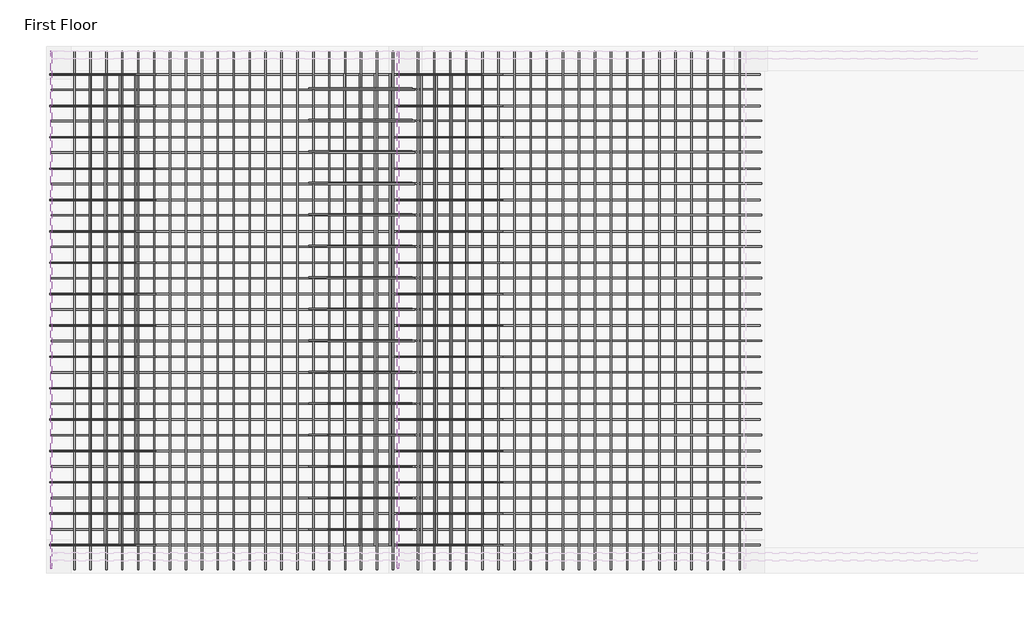
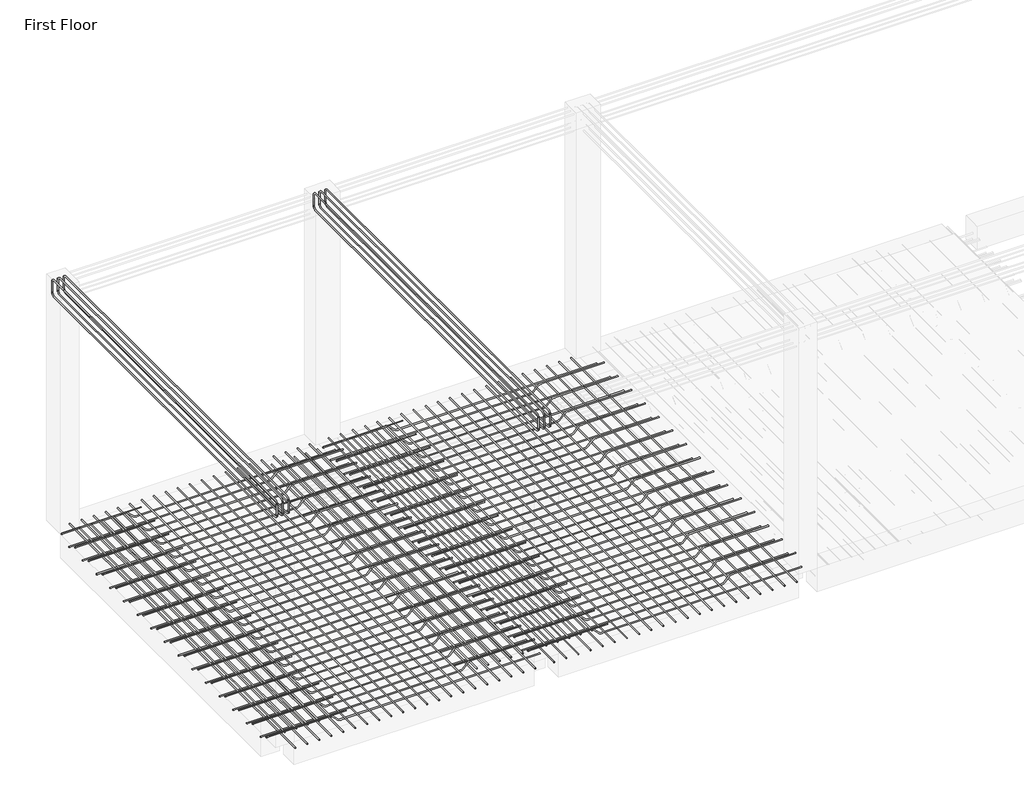
# One storey, part 2 of 4: 16 reinforcing bars.
"""IFC4 building model written with IfcOpenShell, lengths in millimetres."""

from ifc_helpers import new_model, si_unit, point, frame, origin, place, context, project, spatial, polyline, circle_curve, trimmed, segment, composite_curve, source, transform, mapped, element, save
from ifc_brep_helpers import swept_disk

model = new_model("IFC4")

# Units and contexts
model_context = context("Model", 3, world=origin())
ifc_project = project(units=[si_unit("LENGTHUNIT", "METRE", prefix="MILLI")], contexts=[model_context])

# Site, building, storey
site = spatial("IfcSite", under=ifc_project)
building = spatial("IfcBuilding", under=site)
storey = spatial("IfcBuildingStorey", under=building, Name="First Floor", Elevation=3200.4)

# Reinforcing bars
placement = place(None, origin())
reinforcing_bar_shape = source(origin(), model_context, "Body", "SolidModel", [
    swept_disk(composite_curve([segment(polyline([(-9335.8112474, 5017.2334631, 6163.6994949), (-9335.8112474, 5017.2334631, 6311.6994949)]), True, "CONTINUOUS"), segment(trimmed(circle_curve(frame((-9335.8112474, 4971.2334631, 6311.6994949), z_axis=(1.0, 0.0, 0.0), x_axis=(0.0, 46.0, 0.0)), 46.0), [point((-9335.8112474, 5017.2334631, 6311.6994949))], [point((-9335.8112474, 4971.2334631, 6357.6994949))], True, "CARTESIAN"), True, "CONTINUOUS"), segment(polyline([(-9335.8112474, 4971.2334631, 6357.6994949), (-9335.8112474, 278.4334631, 6357.6994949)]), True, "CONTINUOUS"), segment(trimmed(circle_curve(frame((-9335.8112474, 278.4334631, 6311.6994949), z_axis=(1.0, 0.0, 0.0), x_axis=(0.0, 0.0, 46.0)), 46.0), [point((-9335.8112474, 278.4334631, 6357.6994949))], [point((-9335.8112474, 232.4334631, 6311.6994949))], True, "CARTESIAN"), True, "CONTINUOUS"), segment(polyline([(-9335.8112474, 232.4334631, 6311.6994949), (-9335.8112474, 232.4334631, 6163.6994949)]), True, "CONTINUOUS")], self_intersect=False), 6.0),
])
element("IfcReinforcingBar", 1, at=placement, inside=storey, context=model_context, shape_type="MappedRepresentation", body=[
    mapped(reinforcing_bar_shape, transform((0.0, 0.0, 0.0), x_axis=(1.0, 0.0, 0.0), y_axis=(0.0, 1.0, 0.0), z_axis=(0.0, 0.0, 1.0))),
    mapped(reinforcing_bar_shape, transform((71.1994949, 0.0, 0.0), x_axis=(1.0, 0.0, 0.0), y_axis=(0.0, 1.0, 0.0), z_axis=(0.0, 0.0, 1.0))),
    mapped(reinforcing_bar_shape, transform((142.3989899, 0.0, 0.0), x_axis=(1.0, 0.0, 0.0), y_axis=(0.0, 1.0, 0.0), z_axis=(0.0, 0.0, 1.0))),
])
reinforcing_bar_2_shape = source(origin(), model_context, "Body", "SolidModel", [
    swept_disk(composite_curve([segment(polyline([(-9335.8112474, 5017.2334631, 6333.1005051), (-9335.8112474, 5017.2334631, 6185.1005051)]), True, "CONTINUOUS"), segment(trimmed(circle_curve(frame((-9335.8112474, 4971.2334631, 6185.1005051), z_axis=(-1.0, 0.0, 0.0), x_axis=(0.0, 46.0, 0.0)), 46.0), [point((-9335.8112474, 5017.2334631, 6185.1005051))], [point((-9335.8112474, 4971.2334631, 6139.1005051))], True, "CARTESIAN"), True, "CONTINUOUS"), segment(polyline([(-9335.8112474, 4971.2334631, 6139.1005051), (-9335.8112474, 278.4334631, 6139.1005051)]), True, "CONTINUOUS"), segment(trimmed(circle_curve(frame((-9335.8112474, 278.4334631, 6185.1005051), z_axis=(-1.0, 0.0, 0.0), x_axis=(0.0, 0.0, -46.0)), 46.0), [point((-9335.8112474, 278.4334631, 6139.1005051))], [point((-9335.8112474, 232.4334631, 6185.1005051))], True, "CARTESIAN"), True, "CONTINUOUS"), segment(polyline([(-9335.8112474, 232.4334631, 6185.1005051), (-9335.8112474, 232.4334631, 6333.1005051)]), True, "CONTINUOUS")], self_intersect=False), 6.0),
])
element("IfcReinforcingBar", 2, at=placement, inside=storey, context=model_context, shape_type="MappedRepresentation", body=[
    mapped(reinforcing_bar_2_shape, transform((0.0, 0.0, 0.0), x_axis=(1.0, 0.0, 0.0), y_axis=(0.0, 1.0, 0.0), z_axis=(0.0, 0.0, 1.0))),
    mapped(reinforcing_bar_2_shape, transform((71.1994949, 0.0, 0.0), x_axis=(1.0, 0.0, 0.0), y_axis=(0.0, 1.0, 0.0), z_axis=(0.0, 0.0, 1.0))),
    mapped(reinforcing_bar_2_shape, transform((142.3989899, 0.0, 0.0), x_axis=(1.0, 0.0, 0.0), y_axis=(0.0, 1.0, 0.0), z_axis=(0.0, 0.0, 1.0))),
])
reinforcing_bar_3_shape = source(origin(), model_context, "Body", "SolidModel", [
    swept_disk(composite_curve([segment(polyline([(-6122.7112474, 5017.2334631, 6163.6994949), (-6122.7112474, 5017.2334631, 6311.6994949)]), True, "CONTINUOUS"), segment(trimmed(circle_curve(frame((-6122.7112474, 4971.2334631, 6311.6994949), z_axis=(1.0, 0.0, 0.0), x_axis=(0.0, 46.0, 0.0)), 46.0), [point((-6122.7112474, 5017.2334631, 6311.6994949))], [point((-6122.7112474, 4971.2334631, 6357.6994949))], True, "CARTESIAN"), True, "CONTINUOUS"), segment(polyline([(-6122.7112474, 4971.2334631, 6357.6994949), (-6122.7112474, 278.4334631, 6357.6994949)]), True, "CONTINUOUS"), segment(trimmed(circle_curve(frame((-6122.7112474, 278.4334631, 6311.6994949), z_axis=(1.0, 0.0, 0.0), x_axis=(0.0, 0.0, 46.0)), 46.0), [point((-6122.7112474, 278.4334631, 6357.6994949))], [point((-6122.7112474, 232.4334631, 6311.6994949))], True, "CARTESIAN"), True, "CONTINUOUS"), segment(polyline([(-6122.7112474, 232.4334631, 6311.6994949), (-6122.7112474, 232.4334631, 6163.6994949)]), True, "CONTINUOUS")], self_intersect=False), 6.0),
])
element("IfcReinforcingBar", 3, at=placement, inside=storey, context=model_context, shape_type="MappedRepresentation", body=[
    mapped(reinforcing_bar_3_shape, transform((0.0, 0.0, 0.0), x_axis=(1.0, 0.0, 0.0), y_axis=(0.0, 1.0, 0.0), z_axis=(0.0, 0.0, 1.0))),
    mapped(reinforcing_bar_3_shape, transform((71.1994949, 0.0, 0.0), x_axis=(1.0, 0.0, 0.0), y_axis=(0.0, 1.0, 0.0), z_axis=(0.0, 0.0, 1.0))),
    mapped(reinforcing_bar_3_shape, transform((142.3989899, 0.0, 0.0), x_axis=(1.0, 0.0, 0.0), y_axis=(0.0, 1.0, 0.0), z_axis=(0.0, 0.0, 1.0))),
])
reinforcing_bar_4_shape = source(origin(), model_context, "Body", "SolidModel", [
    swept_disk(composite_curve([segment(polyline([(-6122.7112474, 5017.2334631, 6333.1005051), (-6122.7112474, 5017.2334631, 6185.1005051)]), True, "CONTINUOUS"), segment(trimmed(circle_curve(frame((-6122.7112474, 4971.2334631, 6185.1005051), z_axis=(-1.0, 0.0, 0.0), x_axis=(0.0, 46.0, 0.0)), 46.0), [point((-6122.7112474, 5017.2334631, 6185.1005051))], [point((-6122.7112474, 4971.2334631, 6139.1005051))], True, "CARTESIAN"), True, "CONTINUOUS"), segment(polyline([(-6122.7112474, 4971.2334631, 6139.1005051), (-6122.7112474, 278.4334631, 6139.1005051)]), True, "CONTINUOUS"), segment(trimmed(circle_curve(frame((-6122.7112474, 278.4334631, 6185.1005051), z_axis=(-1.0, 0.0, 0.0), x_axis=(0.0, 0.0, -46.0)), 46.0), [point((-6122.7112474, 278.4334631, 6139.1005051))], [point((-6122.7112474, 232.4334631, 6185.1005051))], True, "CARTESIAN"), True, "CONTINUOUS"), segment(polyline([(-6122.7112474, 232.4334631, 6185.1005051), (-6122.7112474, 232.4334631, 6333.1005051)]), True, "CONTINUOUS")], self_intersect=False), 6.0),
])
element("IfcReinforcingBar", 4, at=placement, inside=storey, context=model_context, shape_type="MappedRepresentation", body=[
    mapped(reinforcing_bar_4_shape, transform((0.0, 0.0, 0.0), x_axis=(1.0, 0.0, 0.0), y_axis=(0.0, 1.0, 0.0), z_axis=(0.0, 0.0, 1.0))),
    mapped(reinforcing_bar_4_shape, transform((71.1994949, 0.0, 0.0), x_axis=(1.0, 0.0, 0.0), y_axis=(0.0, 1.0, 0.0), z_axis=(0.0, 0.0, 1.0))),
    mapped(reinforcing_bar_4_shape, transform((142.3989899, 0.0, 0.0), x_axis=(1.0, 0.0, 0.0), y_axis=(0.0, 1.0, 0.0), z_axis=(0.0, 0.0, 1.0))),
])
reinforcing_bar_5_shape = source(origin(), model_context, "Body", "SolidModel", [
    swept_disk(composite_curve([segment(polyline([(-9347.5125695, 4803.6334631, 3169.4), (-8565.5792829, 4803.6334631, 3169.4)]), True, "CONTINUOUS"), segment(trimmed(circle_curve(frame((-8565.5792829, 4803.6334631, 3123.4), z_axis=(0.0, 1.0, 0.0), x_axis=(0.0, 0.0, 46.0)), 46.0), [point((-8565.5792829, 4803.6334631, 3169.4))], [point((-8533.052371, 4803.6334631, 3155.9269119))], True, "CARTESIAN"), True, "CONTINUOUS"), segment(polyline([(-8533.052371, 4803.6334631, 3155.9269119), (-8469.5985471, 4803.6334631, 3092.4730881)]), True, "CONTINUOUS"), segment(trimmed(circle_curve(frame((-8437.0716352, 4803.6334631, 3125.0), z_axis=(0.0, -1.0000000000000002, 0.0), x_axis=(-32.526911900000414, 0.0, -32.52691189999996)), 46.0), [point((-8469.5985471, 4803.6334631, 3092.4730881))], [point((-8437.0716352, 4803.6334631, 3079.0))], True, "CARTESIAN"), True, "CONTINUOUS"), segment(polyline([(-8437.0716352, 4803.6334631, 3079.0), (-5982.0597449, 4803.6334631, 3079.0)]), True, "CONTINUOUS")], self_intersect=False), 6.0),
])
element("IfcReinforcingBar", 5, at=placement, inside=storey, context=model_context, shape_type="MappedRepresentation", body=[
    mapped(reinforcing_bar_5_shape, transform((0.0, 0.0, 0.0), x_axis=(1.0, 0.0, 0.0), y_axis=(0.0, 1.0, 0.0), z_axis=(0.0, 0.0, 1.0))),
    mapped(reinforcing_bar_5_shape, transform((0.0, -290.5066667, 0.0), x_axis=(1.0, 0.0, 0.0), y_axis=(0.0, 1.0, 0.0), z_axis=(0.0, 0.0, 1.0))),
    mapped(reinforcing_bar_5_shape, transform((0.0, -581.0133333, 0.0), x_axis=(1.0, 0.0, 0.0), y_axis=(0.0, 1.0, 0.0), z_axis=(0.0, 0.0, 1.0))),
    mapped(reinforcing_bar_5_shape, transform((0.0, -871.52, 0.0), x_axis=(1.0, 0.0, 0.0), y_axis=(0.0, 1.0, 0.0), z_axis=(0.0, 0.0, 1.0))),
    mapped(reinforcing_bar_5_shape, transform((0.0, -1162.0266667, 0.0), x_axis=(1.0, 0.0, 0.0), y_axis=(0.0, 1.0, 0.0), z_axis=(0.0, 0.0, 1.0))),
    mapped(reinforcing_bar_5_shape, transform((0.0, -1452.5333333, 0.0), x_axis=(1.0, 0.0, 0.0), y_axis=(0.0, 1.0, 0.0), z_axis=(0.0, 0.0, 1.0))),
    mapped(reinforcing_bar_5_shape, transform((0.0, -1743.04, 0.0), x_axis=(1.0, 0.0, 0.0), y_axis=(0.0, 1.0, 0.0), z_axis=(0.0, 0.0, 1.0))),
    mapped(reinforcing_bar_5_shape, transform((0.0, -2033.5466667, 0.0), x_axis=(1.0, 0.0, 0.0), y_axis=(0.0, 1.0, 0.0), z_axis=(0.0, 0.0, 1.0))),
    mapped(reinforcing_bar_5_shape, transform((0.0, -2324.0533333, 0.0), x_axis=(1.0, 0.0, 0.0), y_axis=(0.0, 1.0, 0.0), z_axis=(0.0, 0.0, 1.0))),
    mapped(reinforcing_bar_5_shape, transform((0.0, -2614.56, 0.0), x_axis=(1.0, 0.0, 0.0), y_axis=(0.0, 1.0, 0.0), z_axis=(0.0, 0.0, 1.0))),
    mapped(reinforcing_bar_5_shape, transform((0.0, -2905.0666667, 0.0), x_axis=(1.0, 0.0, 0.0), y_axis=(0.0, 1.0, 0.0), z_axis=(0.0, 0.0, 1.0))),
    mapped(reinforcing_bar_5_shape, transform((0.0, -3195.5733333, 0.0), x_axis=(1.0, 0.0, 0.0), y_axis=(0.0, 1.0, 0.0), z_axis=(0.0, 0.0, 1.0))),
    mapped(reinforcing_bar_5_shape, transform((0.0, -3486.08, 0.0), x_axis=(1.0, 0.0, 0.0), y_axis=(0.0, 1.0, 0.0), z_axis=(0.0, 0.0, 1.0))),
    mapped(reinforcing_bar_5_shape, transform((0.0, -3776.5866667, 0.0), x_axis=(1.0, 0.0, 0.0), y_axis=(0.0, 1.0, 0.0), z_axis=(0.0, 0.0, 1.0))),
    mapped(reinforcing_bar_5_shape, transform((0.0, -4067.0933333, 0.0), x_axis=(1.0, 0.0, 0.0), y_axis=(0.0, 1.0, 0.0), z_axis=(0.0, 0.0, 1.0))),
    mapped(reinforcing_bar_5_shape, transform((0.0, -4357.6, 0.0), x_axis=(1.0, 0.0, 0.0), y_axis=(0.0, 1.0, 0.0), z_axis=(0.0, 0.0, 1.0))),
])
reinforcing_bar_6_shape = source(origin(), model_context, "Body", "SolidModel", [
    swept_disk(composite_curve([segment(polyline([(-5968.6109354, 590.4513536, 3169.4), (-6750.544222, 590.4513536, 3169.4)]), True, "CONTINUOUS"), segment(trimmed(circle_curve(frame((-6750.544222, 590.4513536, 3123.4), z_axis=(0.0, -1.0, 0.0), x_axis=(0.0, 0.0, 46.0)), 46.0), [point((-6750.544222, 590.4513536, 3169.4))], [point((-6783.0711339, 590.4513536, 3155.9269119))], True, "CARTESIAN"), True, "CONTINUOUS"), segment(polyline([(-6783.0711339, 590.4513536, 3155.9269119), (-6846.5249578, 590.4513536, 3092.4730881)]), True, "CONTINUOUS"), segment(trimmed(circle_curve(frame((-6879.0518697, 590.4513536, 3125.0), z_axis=(0.0, 1.0000000000000002, 0.0), x_axis=(32.526911899999504, 0.0, -32.52691189999996)), 46.0), [point((-6846.5249578, 590.4513536, 3092.4730881))], [point((-6879.0518697, 590.4513536, 3079.0))], True, "CARTESIAN"), True, "CONTINUOUS"), segment(polyline([(-6879.0518697, 590.4513536, 3079.0), (-9334.06376, 590.4513536, 3079.0)]), True, "CONTINUOUS")], self_intersect=False), 6.0),
])
element("IfcReinforcingBar", 6, at=placement, inside=storey, context=model_context, shape_type="MappedRepresentation", body=[
    mapped(reinforcing_bar_6_shape, transform((0.0, 0.0, 0.0), x_axis=(1.0, 0.0, 0.0), y_axis=(0.0, 1.0, 0.0), z_axis=(0.0, 0.0, 1.0))),
    mapped(reinforcing_bar_6_shape, transform((0.0, 290.9296088, 0.0), x_axis=(1.0, 0.0, 0.0), y_axis=(0.0, 1.0, 0.0), z_axis=(0.0, 0.0, 1.0))),
    mapped(reinforcing_bar_6_shape, transform((0.0, 581.8592177, 0.0), x_axis=(1.0, 0.0, 0.0), y_axis=(0.0, 1.0, 0.0), z_axis=(0.0, 0.0, 1.0))),
    mapped(reinforcing_bar_6_shape, transform((0.0, 872.7888265, 0.0), x_axis=(1.0, 0.0, 0.0), y_axis=(0.0, 1.0, 0.0), z_axis=(0.0, 0.0, 1.0))),
    mapped(reinforcing_bar_6_shape, transform((0.0, 1163.7184353, 0.0), x_axis=(1.0, 0.0, 0.0), y_axis=(0.0, 1.0, 0.0), z_axis=(0.0, 0.0, 1.0))),
    mapped(reinforcing_bar_6_shape, transform((0.0, 1454.6480442, 0.0), x_axis=(1.0, 0.0, 0.0), y_axis=(0.0, 1.0, 0.0), z_axis=(0.0, 0.0, 1.0))),
    mapped(reinforcing_bar_6_shape, transform((0.0, 1745.577653, 0.0), x_axis=(1.0, 0.0, 0.0), y_axis=(0.0, 1.0, 0.0), z_axis=(0.0, 0.0, 1.0))),
    mapped(reinforcing_bar_6_shape, transform((0.0, 2036.5072618, 0.0), x_axis=(1.0, 0.0, 0.0), y_axis=(0.0, 1.0, 0.0), z_axis=(0.0, 0.0, 1.0))),
    mapped(reinforcing_bar_6_shape, transform((0.0, 2327.4368707, 0.0), x_axis=(1.0, 0.0, 0.0), y_axis=(0.0, 1.0, 0.0), z_axis=(0.0, 0.0, 1.0))),
    mapped(reinforcing_bar_6_shape, transform((0.0, 2618.3664795, 0.0), x_axis=(1.0, 0.0, 0.0), y_axis=(0.0, 1.0, 0.0), z_axis=(0.0, 0.0, 1.0))),
    mapped(reinforcing_bar_6_shape, transform((0.0, 2909.2960883, 0.0), x_axis=(1.0, 0.0, 0.0), y_axis=(0.0, 1.0, 0.0), z_axis=(0.0, 0.0, 1.0))),
    mapped(reinforcing_bar_6_shape, transform((0.0, 3200.2256972, 0.0), x_axis=(1.0, 0.0, 0.0), y_axis=(0.0, 1.0, 0.0), z_axis=(0.0, 0.0, 1.0))),
    mapped(reinforcing_bar_6_shape, transform((0.0, 3491.155306, 0.0), x_axis=(1.0, 0.0, 0.0), y_axis=(0.0, 1.0, 0.0), z_axis=(0.0, 0.0, 1.0))),
    mapped(reinforcing_bar_6_shape, transform((0.0, 3782.0849148, 0.0), x_axis=(1.0, 0.0, 0.0), y_axis=(0.0, 1.0, 0.0), z_axis=(0.0, 0.0, 1.0))),
    mapped(reinforcing_bar_6_shape, transform((0.0, 4073.0145236, 0.0), x_axis=(1.0, 0.0, 0.0), y_axis=(0.0, 1.0, 0.0), z_axis=(0.0, 0.0, 1.0))),
])
reinforcing_bar_7_shape = source(origin(), model_context, "Body", "SolidModel", [
    swept_disk(composite_curve([segment(polyline([(-8556.5984173, 4809.6334631, 3159.1006995), (-8556.5984173, 440.0334631, 3159.1006995)]), True, "CONTINUOUS")], self_intersect=False), 6.0),
])
element("IfcReinforcingBar", 7, at=placement, inside=storey, context=model_context, shape_type="MappedRepresentation", body=[
    mapped(reinforcing_bar_7_shape, transform((0.0, 0.0, 0.0), x_axis=(1.0, 0.0, 0.0), y_axis=(0.0, 1.0, 0.0), z_axis=(0.0, 0.0, 1.0))),
    mapped(reinforcing_bar_7_shape, transform((-140.6783338, 0.0, 0.0), x_axis=(1.0, 0.0, 0.0), y_axis=(0.0, 1.0, 0.0), z_axis=(0.0, 0.0, 1.0))),
    mapped(reinforcing_bar_7_shape, transform((-281.3566676, 0.0, 0.0), x_axis=(1.0, 0.0, 0.0), y_axis=(0.0, 1.0, 0.0), z_axis=(0.0, 0.0, 1.0))),
    mapped(reinforcing_bar_7_shape, transform((-422.0350014, 0.0, 0.0), x_axis=(1.0, 0.0, 0.0), y_axis=(0.0, 1.0, 0.0), z_axis=(0.0, 0.0, 1.0))),
    mapped(reinforcing_bar_7_shape, transform((-562.7133352, 0.0, 0.0), x_axis=(1.0, 0.0, 0.0), y_axis=(0.0, 1.0, 0.0), z_axis=(0.0, 0.0, 1.0))),
])
reinforcing_bar_8_shape = source(origin(), model_context, "Body", "SolidModel", [
    swept_disk(composite_curve([segment(polyline([(-6759.5250876, 4809.6334631, 3159.1006995), (-6759.5250876, 440.0334631, 3159.1006995)]), True, "CONTINUOUS")], self_intersect=False), 6.0),
])
element("IfcReinforcingBar", 8, at=placement, inside=storey, context=model_context, shape_type="MappedRepresentation", body=[
    mapped(reinforcing_bar_8_shape, transform((0.0, 0.0, 0.0), x_axis=(1.0, 0.0, 0.0), y_axis=(0.0, 1.0, 0.0), z_axis=(0.0, 0.0, 1.0))),
    mapped(reinforcing_bar_8_shape, transform((140.6783338, 0.0, 0.0), x_axis=(1.0, 0.0, 0.0), y_axis=(0.0, 1.0, 0.0), z_axis=(0.0, 0.0, 1.0))),
    mapped(reinforcing_bar_8_shape, transform((281.3566676, 0.0, 0.0), x_axis=(1.0, 0.0, 0.0), y_axis=(0.0, 1.0, 0.0), z_axis=(0.0, 0.0, 1.0))),
    mapped(reinforcing_bar_8_shape, transform((422.0350014, 0.0, 0.0), x_axis=(1.0, 0.0, 0.0), y_axis=(0.0, 1.0, 0.0), z_axis=(0.0, 0.0, 1.0))),
    mapped(reinforcing_bar_8_shape, transform((562.7133352, 0.0, 0.0), x_axis=(1.0, 0.0, 0.0), y_axis=(0.0, 1.0, 0.0), z_axis=(0.0, 0.0, 1.0))),
])
reinforcing_bar_9_shape = source(origin(), model_context, "Body", "SolidModel", [
    swept_disk(composite_curve([segment(polyline([(-9338.4522926, 4805.6334631, 3171.4), (-8365.7369752, 4805.6334631, 3171.4)]), True, "CONTINUOUS")], self_intersect=False), 4.0),
])
element("IfcReinforcingBar", 9, at=placement, inside=storey, context=model_context, shape_type="MappedRepresentation", body=[
    mapped(reinforcing_bar_9_shape, transform((0.0, 0.0, 0.0), x_axis=(1.0, 0.0, 0.0), y_axis=(0.0, 1.0, 0.0), z_axis=(0.0, 0.0, 1.0))),
    mapped(reinforcing_bar_9_shape, transform((0.0, -290.7733333, 0.0), x_axis=(1.0, 0.0, 0.0), y_axis=(0.0, 1.0, 0.0), z_axis=(0.0, 0.0, 1.0))),
    mapped(reinforcing_bar_9_shape, transform((0.0, -581.5466667, 0.0), x_axis=(1.0, 0.0, 0.0), y_axis=(0.0, 1.0, 0.0), z_axis=(0.0, 0.0, 1.0))),
    mapped(reinforcing_bar_9_shape, transform((0.0, -872.32, 0.0), x_axis=(1.0, 0.0, 0.0), y_axis=(0.0, 1.0, 0.0), z_axis=(0.0, 0.0, 1.0))),
    mapped(reinforcing_bar_9_shape, transform((0.0, -1163.0933333, 0.0), x_axis=(1.0, 0.0, 0.0), y_axis=(0.0, 1.0, 0.0), z_axis=(0.0, 0.0, 1.0))),
    mapped(reinforcing_bar_9_shape, transform((0.0, -1453.8666667, 0.0), x_axis=(1.0, 0.0, 0.0), y_axis=(0.0, 1.0, 0.0), z_axis=(0.0, 0.0, 1.0))),
    mapped(reinforcing_bar_9_shape, transform((0.0, -1744.64, 0.0), x_axis=(1.0, 0.0, 0.0), y_axis=(0.0, 1.0, 0.0), z_axis=(0.0, 0.0, 1.0))),
    mapped(reinforcing_bar_9_shape, transform((0.0, -2035.4133333, 0.0), x_axis=(1.0, 0.0, 0.0), y_axis=(0.0, 1.0, 0.0), z_axis=(0.0, 0.0, 1.0))),
    mapped(reinforcing_bar_9_shape, transform((0.0, -2326.1866667, 0.0), x_axis=(1.0, 0.0, 0.0), y_axis=(0.0, 1.0, 0.0), z_axis=(0.0, 0.0, 1.0))),
    mapped(reinforcing_bar_9_shape, transform((0.0, -2616.96, 0.0), x_axis=(1.0, 0.0, 0.0), y_axis=(0.0, 1.0, 0.0), z_axis=(0.0, 0.0, 1.0))),
    mapped(reinforcing_bar_9_shape, transform((0.0, -2907.7333333, 0.0), x_axis=(1.0, 0.0, 0.0), y_axis=(0.0, 1.0, 0.0), z_axis=(0.0, 0.0, 1.0))),
    mapped(reinforcing_bar_9_shape, transform((0.0, -3198.5066667, 0.0), x_axis=(1.0, 0.0, 0.0), y_axis=(0.0, 1.0, 0.0), z_axis=(0.0, 0.0, 1.0))),
    mapped(reinforcing_bar_9_shape, transform((0.0, -3489.28, 0.0), x_axis=(1.0, 0.0, 0.0), y_axis=(0.0, 1.0, 0.0), z_axis=(0.0, 0.0, 1.0))),
    mapped(reinforcing_bar_9_shape, transform((0.0, -3780.0533333, 0.0), x_axis=(1.0, 0.0, 0.0), y_axis=(0.0, 1.0, 0.0), z_axis=(0.0, 0.0, 1.0))),
    mapped(reinforcing_bar_9_shape, transform((0.0, -4070.8266667, 0.0), x_axis=(1.0, 0.0, 0.0), y_axis=(0.0, 1.0, 0.0), z_axis=(0.0, 0.0, 1.0))),
    mapped(reinforcing_bar_9_shape, transform((0.0, -4361.6, 0.0), x_axis=(1.0, 0.0, 0.0), y_axis=(0.0, 1.0, 0.0), z_axis=(0.0, 0.0, 1.0))),
])
reinforcing_bar_10_shape = source(origin(), model_context, "Body", "SolidModel", [
    swept_disk(composite_curve([segment(polyline([(-5991.3123639, 4678.4115375, 3171.4), (-6950.3865297, 4678.4115375, 3171.4)]), True, "CONTINUOUS")], self_intersect=False), 4.0),
])
element("IfcReinforcingBar", 10, at=placement, inside=storey, context=model_context, shape_type="MappedRepresentation", body=[
    mapped(reinforcing_bar_10_shape, transform((0.0, 0.0, 0.0), x_axis=(1.0, 0.0, 0.0), y_axis=(0.0, 1.0, 0.0), z_axis=(0.0, 0.0, 1.0))),
    mapped(reinforcing_bar_10_shape, transform((0.0, -291.8025106, 0.0), x_axis=(1.0, 0.0, 0.0), y_axis=(0.0, 1.0, 0.0), z_axis=(0.0, 0.0, 1.0))),
    mapped(reinforcing_bar_10_shape, transform((0.0, -583.6050212, 0.0), x_axis=(1.0, 0.0, 0.0), y_axis=(0.0, 1.0, 0.0), z_axis=(0.0, 0.0, 1.0))),
    mapped(reinforcing_bar_10_shape, transform((0.0, -875.4075319, 0.0), x_axis=(1.0, 0.0, 0.0), y_axis=(0.0, 1.0, 0.0), z_axis=(0.0, 0.0, 1.0))),
    mapped(reinforcing_bar_10_shape, transform((0.0, -1167.2100425, 0.0), x_axis=(1.0, 0.0, 0.0), y_axis=(0.0, 1.0, 0.0), z_axis=(0.0, 0.0, 1.0))),
    mapped(reinforcing_bar_10_shape, transform((0.0, -1459.0125531, 0.0), x_axis=(1.0, 0.0, 0.0), y_axis=(0.0, 1.0, 0.0), z_axis=(0.0, 0.0, 1.0))),
    mapped(reinforcing_bar_10_shape, transform((0.0, -1750.8150637, 0.0), x_axis=(1.0, 0.0, 0.0), y_axis=(0.0, 1.0, 0.0), z_axis=(0.0, 0.0, 1.0))),
    mapped(reinforcing_bar_10_shape, transform((0.0, -2042.6175743, 0.0), x_axis=(1.0, 0.0, 0.0), y_axis=(0.0, 1.0, 0.0), z_axis=(0.0, 0.0, 1.0))),
    mapped(reinforcing_bar_10_shape, transform((0.0, -2334.420085, 0.0), x_axis=(1.0, 0.0, 0.0), y_axis=(0.0, 1.0, 0.0), z_axis=(0.0, 0.0, 1.0))),
    mapped(reinforcing_bar_10_shape, transform((0.0, -2626.2225956, 0.0), x_axis=(1.0, 0.0, 0.0), y_axis=(0.0, 1.0, 0.0), z_axis=(0.0, 0.0, 1.0))),
    mapped(reinforcing_bar_10_shape, transform((0.0, -2918.0251062, 0.0), x_axis=(1.0, 0.0, 0.0), y_axis=(0.0, 1.0, 0.0), z_axis=(0.0, 0.0, 1.0))),
    mapped(reinforcing_bar_10_shape, transform((0.0, -3209.8276168, 0.0), x_axis=(1.0, 0.0, 0.0), y_axis=(0.0, 1.0, 0.0), z_axis=(0.0, 0.0, 1.0))),
    mapped(reinforcing_bar_10_shape, transform((0.0, -3501.6301274, 0.0), x_axis=(1.0, 0.0, 0.0), y_axis=(0.0, 1.0, 0.0), z_axis=(0.0, 0.0, 1.0))),
    mapped(reinforcing_bar_10_shape, transform((0.0, -3793.4326381, 0.0), x_axis=(1.0, 0.0, 0.0), y_axis=(0.0, 1.0, 0.0), z_axis=(0.0, 0.0, 1.0))),
    mapped(reinforcing_bar_10_shape, transform((0.0, -4085.2351487, 0.0), x_axis=(1.0, 0.0, 0.0), y_axis=(0.0, 1.0, 0.0), z_axis=(0.0, 0.0, 1.0))),
])
reinforcing_bar_11_shape = source(origin(), model_context, "Body", "SolidModel", [
    swept_disk(composite_curve([segment(polyline([(-6169.8117524, 218.9117605, 3087.5387401), (-6169.8117524, 5019.9992064, 3087.5387401)]), True, "CONTINUOUS")], self_intersect=False), 6.0),
])
element("IfcReinforcingBar", 11, at=placement, inside=storey, context=model_context, shape_type="MappedRepresentation", body=[
    mapped(reinforcing_bar_11_shape, transform((0.0, 0.0, 0.0), x_axis=(1.0, 0.0, 0.0), y_axis=(0.0, 1.0, 0.0), z_axis=(0.0, 0.0, 1.0))),
    mapped(reinforcing_bar_11_shape, transform((-147.475, 0.0, 0.0), x_axis=(1.0, 0.0, 0.0), y_axis=(0.0, 1.0, 0.0), z_axis=(0.0, 0.0, 1.0))),
    mapped(reinforcing_bar_11_shape, transform((-294.95, 0.0, 0.0), x_axis=(1.0, 0.0, 0.0), y_axis=(0.0, 1.0, 0.0), z_axis=(0.0, 0.0, 1.0))),
    mapped(reinforcing_bar_11_shape, transform((-442.425, 0.0, 0.0), x_axis=(1.0, 0.0, 0.0), y_axis=(0.0, 1.0, 0.0), z_axis=(0.0, 0.0, 1.0))),
    mapped(reinforcing_bar_11_shape, transform((-589.9, 0.0, 0.0), x_axis=(1.0, 0.0, 0.0), y_axis=(0.0, 1.0, 0.0), z_axis=(0.0, 0.0, 1.0))),
    mapped(reinforcing_bar_11_shape, transform((-737.375, 0.0, 0.0), x_axis=(1.0, 0.0, 0.0), y_axis=(0.0, 1.0, 0.0), z_axis=(0.0, 0.0, 1.0))),
    mapped(reinforcing_bar_11_shape, transform((-884.85, 0.0, 0.0), x_axis=(1.0, 0.0, 0.0), y_axis=(0.0, 1.0, 0.0), z_axis=(0.0, 0.0, 1.0))),
    mapped(reinforcing_bar_11_shape, transform((-1032.325, 0.0, 0.0), x_axis=(1.0, 0.0, 0.0), y_axis=(0.0, 1.0, 0.0), z_axis=(0.0, 0.0, 1.0))),
    mapped(reinforcing_bar_11_shape, transform((-1179.8, 0.0, 0.0), x_axis=(1.0, 0.0, 0.0), y_axis=(0.0, 1.0, 0.0), z_axis=(0.0, 0.0, 1.0))),
    mapped(reinforcing_bar_11_shape, transform((-1327.275, 0.0, 0.0), x_axis=(1.0, 0.0, 0.0), y_axis=(0.0, 1.0, 0.0), z_axis=(0.0, 0.0, 1.0))),
    mapped(reinforcing_bar_11_shape, transform((-1474.75, 0.0, 0.0), x_axis=(1.0, 0.0, 0.0), y_axis=(0.0, 1.0, 0.0), z_axis=(0.0, 0.0, 1.0))),
    mapped(reinforcing_bar_11_shape, transform((-1622.225, 0.0, 0.0), x_axis=(1.0, 0.0, 0.0), y_axis=(0.0, 1.0, 0.0), z_axis=(0.0, 0.0, 1.0))),
    mapped(reinforcing_bar_11_shape, transform((-1769.7, 0.0, 0.0), x_axis=(1.0, 0.0, 0.0), y_axis=(0.0, 1.0, 0.0), z_axis=(0.0, 0.0, 1.0))),
    mapped(reinforcing_bar_11_shape, transform((-1917.175, 0.0, 0.0), x_axis=(1.0, 0.0, 0.0), y_axis=(0.0, 1.0, 0.0), z_axis=(0.0, 0.0, 1.0))),
    mapped(reinforcing_bar_11_shape, transform((-2064.65, 0.0, 0.0), x_axis=(1.0, 0.0, 0.0), y_axis=(0.0, 1.0, 0.0), z_axis=(0.0, 0.0, 1.0))),
    mapped(reinforcing_bar_11_shape, transform((-2212.125, 0.0, 0.0), x_axis=(1.0, 0.0, 0.0), y_axis=(0.0, 1.0, 0.0), z_axis=(0.0, 0.0, 1.0))),
    mapped(reinforcing_bar_11_shape, transform((-2359.6, 0.0, 0.0), x_axis=(1.0, 0.0, 0.0), y_axis=(0.0, 1.0, 0.0), z_axis=(0.0, 0.0, 1.0))),
    mapped(reinforcing_bar_11_shape, transform((-2507.075, 0.0, 0.0), x_axis=(1.0, 0.0, 0.0), y_axis=(0.0, 1.0, 0.0), z_axis=(0.0, 0.0, 1.0))),
    mapped(reinforcing_bar_11_shape, transform((-2654.55, 0.0, 0.0), x_axis=(1.0, 0.0, 0.0), y_axis=(0.0, 1.0, 0.0), z_axis=(0.0, 0.0, 1.0))),
    mapped(reinforcing_bar_11_shape, transform((-2802.025, 0.0, 0.0), x_axis=(1.0, 0.0, 0.0), y_axis=(0.0, 1.0, 0.0), z_axis=(0.0, 0.0, 1.0))),
    mapped(reinforcing_bar_11_shape, transform((-2949.5, 0.0, 0.0), x_axis=(1.0, 0.0, 0.0), y_axis=(0.0, 1.0, 0.0), z_axis=(0.0, 0.0, 1.0))),
])
reinforcing_bar_12_shape = source(origin(), model_context, "Body", "SolidModel", [
    swept_disk(composite_curve([segment(polyline([(-6134.4125695, 4803.6334631, 3169.4), (-5352.4792829, 4803.6334631, 3169.4)]), True, "CONTINUOUS"), segment(trimmed(circle_curve(frame((-5352.4792829, 4803.6334631, 3123.4), z_axis=(0.0, 1.0, 0.0), x_axis=(0.0, 0.0, 46.0)), 46.0), [point((-5352.4792829, 4803.6334631, 3169.4))], [point((-5319.952371, 4803.6334631, 3155.9269119))], True, "CARTESIAN"), True, "CONTINUOUS"), segment(polyline([(-5319.952371, 4803.6334631, 3155.9269119), (-5256.4985471, 4803.6334631, 3092.4730881)]), True, "CONTINUOUS"), segment(trimmed(circle_curve(frame((-5223.9716352, 4803.6334631, 3125.0), z_axis=(0.0, -1.0000000000000002, 0.0), x_axis=(-32.526911900000414, 0.0, -32.52691189999996)), 46.0), [point((-5256.4985471, 4803.6334631, 3092.4730881))], [point((-5223.9716352, 4803.6334631, 3079.0))], True, "CARTESIAN"), True, "CONTINUOUS"), segment(polyline([(-5223.9716352, 4803.6334631, 3079.0), (-2768.9597449, 4803.6334631, 3079.0)]), True, "CONTINUOUS")], self_intersect=False), 6.0),
])
element("IfcReinforcingBar", 12, at=placement, inside=storey, context=model_context, shape_type="MappedRepresentation", body=[
    mapped(reinforcing_bar_12_shape, transform((0.0, 0.0, 0.0), x_axis=(1.0, 0.0, 0.0), y_axis=(0.0, 1.0, 0.0), z_axis=(0.0, 0.0, 1.0))),
    mapped(reinforcing_bar_12_shape, transform((0.0, -290.5066667, 0.0), x_axis=(1.0, 0.0, 0.0), y_axis=(0.0, 1.0, 0.0), z_axis=(0.0, 0.0, 1.0))),
    mapped(reinforcing_bar_12_shape, transform((0.0, -581.0133333, 0.0), x_axis=(1.0, 0.0, 0.0), y_axis=(0.0, 1.0, 0.0), z_axis=(0.0, 0.0, 1.0))),
    mapped(reinforcing_bar_12_shape, transform((0.0, -871.52, 0.0), x_axis=(1.0, 0.0, 0.0), y_axis=(0.0, 1.0, 0.0), z_axis=(0.0, 0.0, 1.0))),
    mapped(reinforcing_bar_12_shape, transform((0.0, -1162.0266667, 0.0), x_axis=(1.0, 0.0, 0.0), y_axis=(0.0, 1.0, 0.0), z_axis=(0.0, 0.0, 1.0))),
    mapped(reinforcing_bar_12_shape, transform((0.0, -1452.5333333, 0.0), x_axis=(1.0, 0.0, 0.0), y_axis=(0.0, 1.0, 0.0), z_axis=(0.0, 0.0, 1.0))),
    mapped(reinforcing_bar_12_shape, transform((0.0, -1743.04, 0.0), x_axis=(1.0, 0.0, 0.0), y_axis=(0.0, 1.0, 0.0), z_axis=(0.0, 0.0, 1.0))),
    mapped(reinforcing_bar_12_shape, transform((0.0, -2033.5466667, 0.0), x_axis=(1.0, 0.0, 0.0), y_axis=(0.0, 1.0, 0.0), z_axis=(0.0, 0.0, 1.0))),
    mapped(reinforcing_bar_12_shape, transform((0.0, -2324.0533333, 0.0), x_axis=(1.0, 0.0, 0.0), y_axis=(0.0, 1.0, 0.0), z_axis=(0.0, 0.0, 1.0))),
    mapped(reinforcing_bar_12_shape, transform((0.0, -2614.56, 0.0), x_axis=(1.0, 0.0, 0.0), y_axis=(0.0, 1.0, 0.0), z_axis=(0.0, 0.0, 1.0))),
    mapped(reinforcing_bar_12_shape, transform((0.0, -2905.0666667, 0.0), x_axis=(1.0, 0.0, 0.0), y_axis=(0.0, 1.0, 0.0), z_axis=(0.0, 0.0, 1.0))),
    mapped(reinforcing_bar_12_shape, transform((0.0, -3195.5733333, 0.0), x_axis=(1.0, 0.0, 0.0), y_axis=(0.0, 1.0, 0.0), z_axis=(0.0, 0.0, 1.0))),
    mapped(reinforcing_bar_12_shape, transform((0.0, -3486.08, 0.0), x_axis=(1.0, 0.0, 0.0), y_axis=(0.0, 1.0, 0.0), z_axis=(0.0, 0.0, 1.0))),
    mapped(reinforcing_bar_12_shape, transform((0.0, -3776.5866667, 0.0), x_axis=(1.0, 0.0, 0.0), y_axis=(0.0, 1.0, 0.0), z_axis=(0.0, 0.0, 1.0))),
    mapped(reinforcing_bar_12_shape, transform((0.0, -4067.0933333, 0.0), x_axis=(1.0, 0.0, 0.0), y_axis=(0.0, 1.0, 0.0), z_axis=(0.0, 0.0, 1.0))),
    mapped(reinforcing_bar_12_shape, transform((0.0, -4357.6, 0.0), x_axis=(1.0, 0.0, 0.0), y_axis=(0.0, 1.0, 0.0), z_axis=(0.0, 0.0, 1.0))),
])
reinforcing_bar_13_shape = source(origin(), model_context, "Body", "SolidModel", [
    swept_disk(composite_curve([segment(polyline([(-2755.5109354, 590.4513536, 3169.4), (-3537.444222, 590.4513536, 3169.4)]), True, "CONTINUOUS"), segment(trimmed(circle_curve(frame((-3537.444222, 590.4513536, 3123.4), z_axis=(0.0, -1.0, 0.0), x_axis=(0.0, 0.0, 46.0)), 46.0), [point((-3537.444222, 590.4513536, 3169.4))], [point((-3569.9711339, 590.4513536, 3155.9269119))], True, "CARTESIAN"), True, "CONTINUOUS"), segment(polyline([(-3569.9711339, 590.4513536, 3155.9269119), (-3633.4249578, 590.4513536, 3092.4730881)]), True, "CONTINUOUS"), segment(trimmed(circle_curve(frame((-3665.9518697, 590.4513536, 3125.0), z_axis=(0.0, 1.0000000000000002, 0.0), x_axis=(32.52691189999996, 0.0, -32.52691189999996)), 46.0), [point((-3633.4249578, 590.4513536, 3092.4730881))], [point((-3665.9518697, 590.4513536, 3079.0))], True, "CARTESIAN"), True, "CONTINUOUS"), segment(polyline([(-3665.9518697, 590.4513536, 3079.0), (-6120.96376, 590.4513536, 3079.0)]), True, "CONTINUOUS")], self_intersect=False), 6.0),
])
element("IfcReinforcingBar", 13, at=placement, inside=storey, context=model_context, shape_type="MappedRepresentation", body=[
    mapped(reinforcing_bar_13_shape, transform((0.0, 0.0, 0.0), x_axis=(1.0, 0.0, 0.0), y_axis=(0.0, 1.0, 0.0), z_axis=(0.0, 0.0, 1.0))),
    mapped(reinforcing_bar_13_shape, transform((0.0, 291.2629007, 0.0), x_axis=(1.0, 0.0, 0.0), y_axis=(0.0, 1.0, 0.0), z_axis=(0.0, 0.0, 1.0))),
    mapped(reinforcing_bar_13_shape, transform((0.0, 582.5258014, 0.0), x_axis=(1.0, 0.0, 0.0), y_axis=(0.0, 1.0, 0.0), z_axis=(0.0, 0.0, 1.0))),
    mapped(reinforcing_bar_13_shape, transform((0.0, 873.7887021, 0.0), x_axis=(1.0, 0.0, 0.0), y_axis=(0.0, 1.0, 0.0), z_axis=(0.0, 0.0, 1.0))),
    mapped(reinforcing_bar_13_shape, transform((0.0, 1165.0516028, 0.0), x_axis=(1.0, 0.0, 0.0), y_axis=(0.0, 1.0, 0.0), z_axis=(0.0, 0.0, 1.0))),
    mapped(reinforcing_bar_13_shape, transform((0.0, 1456.3145035, 0.0), x_axis=(1.0, 0.0, 0.0), y_axis=(0.0, 1.0, 0.0), z_axis=(0.0, 0.0, 1.0))),
    mapped(reinforcing_bar_13_shape, transform((0.0, 1747.5774042, 0.0), x_axis=(1.0, 0.0, 0.0), y_axis=(0.0, 1.0, 0.0), z_axis=(0.0, 0.0, 1.0))),
    mapped(reinforcing_bar_13_shape, transform((0.0, 2038.8403049, 0.0), x_axis=(1.0, 0.0, 0.0), y_axis=(0.0, 1.0, 0.0), z_axis=(0.0, 0.0, 1.0))),
    mapped(reinforcing_bar_13_shape, transform((0.0, 2330.1032056, 0.0), x_axis=(1.0, 0.0, 0.0), y_axis=(0.0, 1.0, 0.0), z_axis=(0.0, 0.0, 1.0))),
    mapped(reinforcing_bar_13_shape, transform((0.0, 2621.3661063, 0.0), x_axis=(1.0, 0.0, 0.0), y_axis=(0.0, 1.0, 0.0), z_axis=(0.0, 0.0, 1.0))),
    mapped(reinforcing_bar_13_shape, transform((0.0, 2912.629007, 0.0), x_axis=(1.0, 0.0, 0.0), y_axis=(0.0, 1.0, 0.0), z_axis=(0.0, 0.0, 1.0))),
    mapped(reinforcing_bar_13_shape, transform((0.0, 3203.8919077, 0.0), x_axis=(1.0, 0.0, 0.0), y_axis=(0.0, 1.0, 0.0), z_axis=(0.0, 0.0, 1.0))),
    mapped(reinforcing_bar_13_shape, transform((0.0, 3495.1548084, 0.0), x_axis=(1.0, 0.0, 0.0), y_axis=(0.0, 1.0, 0.0), z_axis=(0.0, 0.0, 1.0))),
    mapped(reinforcing_bar_13_shape, transform((0.0, 3786.4177091, 0.0), x_axis=(1.0, 0.0, 0.0), y_axis=(0.0, 1.0, 0.0), z_axis=(0.0, 0.0, 1.0))),
    mapped(reinforcing_bar_13_shape, transform((0.0, 4077.6806098, 0.0), x_axis=(1.0, 0.0, 0.0), y_axis=(0.0, 1.0, 0.0), z_axis=(0.0, 0.0, 1.0))),
])
reinforcing_bar_14_shape = source(origin(), model_context, "Body", "SolidModel", [
    swept_disk(composite_curve([segment(polyline([(-6125.3522926, 4805.6334631, 3171.4), (-5152.6369752, 4805.6334631, 3171.4)]), True, "CONTINUOUS")], self_intersect=False), 4.0),
])
element("IfcReinforcingBar", 14, at=placement, inside=storey, context=model_context, shape_type="MappedRepresentation", body=[
    mapped(reinforcing_bar_14_shape, transform((0.0, 0.0, 0.0), x_axis=(1.0, 0.0, 0.0), y_axis=(0.0, 1.0, 0.0), z_axis=(0.0, 0.0, 1.0))),
    mapped(reinforcing_bar_14_shape, transform((0.0, -290.7733333, 0.0), x_axis=(1.0, 0.0, 0.0), y_axis=(0.0, 1.0, 0.0), z_axis=(0.0, 0.0, 1.0))),
    mapped(reinforcing_bar_14_shape, transform((0.0, -581.5466667, 0.0), x_axis=(1.0, 0.0, 0.0), y_axis=(0.0, 1.0, 0.0), z_axis=(0.0, 0.0, 1.0))),
    mapped(reinforcing_bar_14_shape, transform((0.0, -872.32, 0.0), x_axis=(1.0, 0.0, 0.0), y_axis=(0.0, 1.0, 0.0), z_axis=(0.0, 0.0, 1.0))),
    mapped(reinforcing_bar_14_shape, transform((0.0, -1163.0933333, 0.0), x_axis=(1.0, 0.0, 0.0), y_axis=(0.0, 1.0, 0.0), z_axis=(0.0, 0.0, 1.0))),
    mapped(reinforcing_bar_14_shape, transform((0.0, -1453.8666667, 0.0), x_axis=(1.0, 0.0, 0.0), y_axis=(0.0, 1.0, 0.0), z_axis=(0.0, 0.0, 1.0))),
    mapped(reinforcing_bar_14_shape, transform((0.0, -1744.64, 0.0), x_axis=(1.0, 0.0, 0.0), y_axis=(0.0, 1.0, 0.0), z_axis=(0.0, 0.0, 1.0))),
    mapped(reinforcing_bar_14_shape, transform((0.0, -2035.4133333, 0.0), x_axis=(1.0, 0.0, 0.0), y_axis=(0.0, 1.0, 0.0), z_axis=(0.0, 0.0, 1.0))),
    mapped(reinforcing_bar_14_shape, transform((0.0, -2326.1866667, 0.0), x_axis=(1.0, 0.0, 0.0), y_axis=(0.0, 1.0, 0.0), z_axis=(0.0, 0.0, 1.0))),
    mapped(reinforcing_bar_14_shape, transform((0.0, -2616.96, 0.0), x_axis=(1.0, 0.0, 0.0), y_axis=(0.0, 1.0, 0.0), z_axis=(0.0, 0.0, 1.0))),
    mapped(reinforcing_bar_14_shape, transform((0.0, -2907.7333333, 0.0), x_axis=(1.0, 0.0, 0.0), y_axis=(0.0, 1.0, 0.0), z_axis=(0.0, 0.0, 1.0))),
    mapped(reinforcing_bar_14_shape, transform((0.0, -3198.5066667, 0.0), x_axis=(1.0, 0.0, 0.0), y_axis=(0.0, 1.0, 0.0), z_axis=(0.0, 0.0, 1.0))),
    mapped(reinforcing_bar_14_shape, transform((0.0, -3489.28, 0.0), x_axis=(1.0, 0.0, 0.0), y_axis=(0.0, 1.0, 0.0), z_axis=(0.0, 0.0, 1.0))),
    mapped(reinforcing_bar_14_shape, transform((0.0, -3780.0533333, 0.0), x_axis=(1.0, 0.0, 0.0), y_axis=(0.0, 1.0, 0.0), z_axis=(0.0, 0.0, 1.0))),
    mapped(reinforcing_bar_14_shape, transform((0.0, -4070.8266667, 0.0), x_axis=(1.0, 0.0, 0.0), y_axis=(0.0, 1.0, 0.0), z_axis=(0.0, 0.0, 1.0))),
    mapped(reinforcing_bar_14_shape, transform((0.0, -4361.6, 0.0), x_axis=(1.0, 0.0, 0.0), y_axis=(0.0, 1.0, 0.0), z_axis=(0.0, 0.0, 1.0))),
])
reinforcing_bar_15_shape = source(origin(), model_context, "Body", "SolidModel", [
    swept_disk(composite_curve([segment(polyline([(-2956.7117524, 218.9117605, 3087.5387401), (-2956.7117524, 5019.9992064, 3087.5387401)]), True, "CONTINUOUS")], self_intersect=False), 6.0),
])
element("IfcReinforcingBar", 15, at=placement, inside=storey, context=model_context, shape_type="MappedRepresentation", body=[
    mapped(reinforcing_bar_15_shape, transform((0.0, 0.0, 0.0), x_axis=(1.0, 0.0, 0.0), y_axis=(0.0, 1.0, 0.0), z_axis=(0.0, 0.0, 1.0))),
    mapped(reinforcing_bar_15_shape, transform((-149.025, 0.0, 0.0), x_axis=(1.0, 0.0, 0.0), y_axis=(0.0, 1.0, 0.0), z_axis=(0.0, 0.0, 1.0))),
    mapped(reinforcing_bar_15_shape, transform((-298.05, 0.0, 0.0), x_axis=(1.0, 0.0, 0.0), y_axis=(0.0, 1.0, 0.0), z_axis=(0.0, 0.0, 1.0))),
    mapped(reinforcing_bar_15_shape, transform((-447.075, 0.0, 0.0), x_axis=(1.0, 0.0, 0.0), y_axis=(0.0, 1.0, 0.0), z_axis=(0.0, 0.0, 1.0))),
    mapped(reinforcing_bar_15_shape, transform((-596.1, 0.0, 0.0), x_axis=(1.0, 0.0, 0.0), y_axis=(0.0, 1.0, 0.0), z_axis=(0.0, 0.0, 1.0))),
    mapped(reinforcing_bar_15_shape, transform((-745.125, 0.0, 0.0), x_axis=(1.0, 0.0, 0.0), y_axis=(0.0, 1.0, 0.0), z_axis=(0.0, 0.0, 1.0))),
    mapped(reinforcing_bar_15_shape, transform((-894.15, 0.0, 0.0), x_axis=(1.0, 0.0, 0.0), y_axis=(0.0, 1.0, 0.0), z_axis=(0.0, 0.0, 1.0))),
    mapped(reinforcing_bar_15_shape, transform((-1043.175, 0.0, 0.0), x_axis=(1.0, 0.0, 0.0), y_axis=(0.0, 1.0, 0.0), z_axis=(0.0, 0.0, 1.0))),
    mapped(reinforcing_bar_15_shape, transform((-1192.2, 0.0, 0.0), x_axis=(1.0, 0.0, 0.0), y_axis=(0.0, 1.0, 0.0), z_axis=(0.0, 0.0, 1.0))),
    mapped(reinforcing_bar_15_shape, transform((-1341.225, 0.0, 0.0), x_axis=(1.0, 0.0, 0.0), y_axis=(0.0, 1.0, 0.0), z_axis=(0.0, 0.0, 1.0))),
    mapped(reinforcing_bar_15_shape, transform((-1490.25, 0.0, 0.0), x_axis=(1.0, 0.0, 0.0), y_axis=(0.0, 1.0, 0.0), z_axis=(0.0, 0.0, 1.0))),
    mapped(reinforcing_bar_15_shape, transform((-1639.275, 0.0, 0.0), x_axis=(1.0, 0.0, 0.0), y_axis=(0.0, 1.0, 0.0), z_axis=(0.0, 0.0, 1.0))),
    mapped(reinforcing_bar_15_shape, transform((-1788.3, 0.0, 0.0), x_axis=(1.0, 0.0, 0.0), y_axis=(0.0, 1.0, 0.0), z_axis=(0.0, 0.0, 1.0))),
    mapped(reinforcing_bar_15_shape, transform((-1937.325, 0.0, 0.0), x_axis=(1.0, 0.0, 0.0), y_axis=(0.0, 1.0, 0.0), z_axis=(0.0, 0.0, 1.0))),
    mapped(reinforcing_bar_15_shape, transform((-2086.35, 0.0, 0.0), x_axis=(1.0, 0.0, 0.0), y_axis=(0.0, 1.0, 0.0), z_axis=(0.0, 0.0, 1.0))),
    mapped(reinforcing_bar_15_shape, transform((-2235.375, 0.0, 0.0), x_axis=(1.0, 0.0, 0.0), y_axis=(0.0, 1.0, 0.0), z_axis=(0.0, 0.0, 1.0))),
    mapped(reinforcing_bar_15_shape, transform((-2384.4, 0.0, 0.0), x_axis=(1.0, 0.0, 0.0), y_axis=(0.0, 1.0, 0.0), z_axis=(0.0, 0.0, 1.0))),
    mapped(reinforcing_bar_15_shape, transform((-2533.425, 0.0, 0.0), x_axis=(1.0, 0.0, 0.0), y_axis=(0.0, 1.0, 0.0), z_axis=(0.0, 0.0, 1.0))),
    mapped(reinforcing_bar_15_shape, transform((-2682.45, 0.0, 0.0), x_axis=(1.0, 0.0, 0.0), y_axis=(0.0, 1.0, 0.0), z_axis=(0.0, 0.0, 1.0))),
    mapped(reinforcing_bar_15_shape, transform((-2831.475, 0.0, 0.0), x_axis=(1.0, 0.0, 0.0), y_axis=(0.0, 1.0, 0.0), z_axis=(0.0, 0.0, 1.0))),
    mapped(reinforcing_bar_15_shape, transform((-2980.5, 0.0, 0.0), x_axis=(1.0, 0.0, 0.0), y_axis=(0.0, 1.0, 0.0), z_axis=(0.0, 0.0, 1.0))),
])
reinforcing_bar_16_shape = source(origin(), model_context, "Body", "SolidModel", [
    swept_disk(composite_curve([segment(polyline([(-5343.4984173, 4809.6334631, 3159.1006995), (-5343.4984173, 440.0334631, 3159.1006995)]), True, "CONTINUOUS")], self_intersect=False), 6.0),
])
element("IfcReinforcingBar", 16, at=placement, inside=storey, context=model_context, shape_type="MappedRepresentation", body=[
    mapped(reinforcing_bar_16_shape, transform((0.0, 0.0, 0.0), x_axis=(1.0, 0.0, 0.0), y_axis=(0.0, 1.0, 0.0), z_axis=(0.0, 0.0, 1.0))),
    mapped(reinforcing_bar_16_shape, transform((-140.6783338, 0.0, 0.0), x_axis=(1.0, 0.0, 0.0), y_axis=(0.0, 1.0, 0.0), z_axis=(0.0, 0.0, 1.0))),
    mapped(reinforcing_bar_16_shape, transform((-281.3566676, 0.0, 0.0), x_axis=(1.0, 0.0, 0.0), y_axis=(0.0, 1.0, 0.0), z_axis=(0.0, 0.0, 1.0))),
    mapped(reinforcing_bar_16_shape, transform((-422.0350014, 0.0, 0.0), x_axis=(1.0, 0.0, 0.0), y_axis=(0.0, 1.0, 0.0), z_axis=(0.0, 0.0, 1.0))),
    mapped(reinforcing_bar_16_shape, transform((-562.7133352, 0.0, 0.0), x_axis=(1.0, 0.0, 0.0), y_axis=(0.0, 1.0, 0.0), z_axis=(0.0, 0.0, 1.0))),
])

save(model, "model.ifc")

# Revit data of these elements
# Elements 1, 2, 3, 4, 5, 6, 7, 8, 9, 10, 11, 12, 13, 14, 15, 16 (IfcReinforcingBar)
#   Phase Created = New Construction
